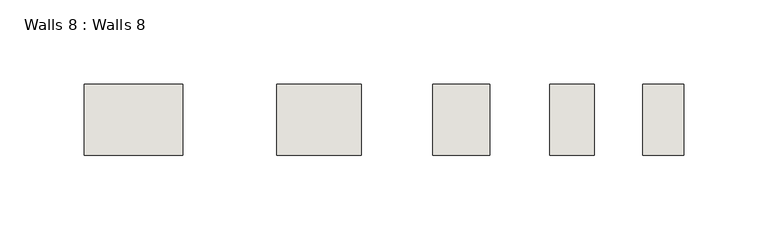
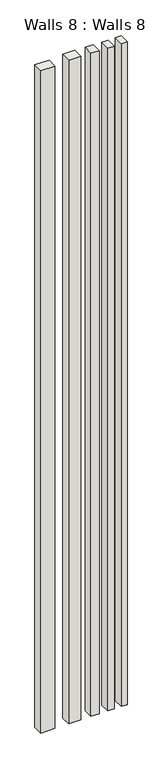
"""IFC4 building model written with IfcOpenShell, lengths in millimetres: wall geometry, Walls 8 : Walls 8."""

from ifc_helpers import new_model, si_unit, frame, origin, place, context, project, spatial, polyline, outline, extrude, source, transform, mapped, element, save


def walls_8_walls_8_e14edf94(model_context):
    return source(origin(), model_context, "Body", "SweptSolid", [
        extrude(outline(polyline([(-6662.2743282, -7775.4794447), (-6686.7552794, -7775.4794447), (-6686.7552794, -7733.3103215), (-6662.2743282, -7733.3103215), (-6662.2743282, -7775.4794447)])), frame((0.0, 0.0, 2899.4015195), z_axis=(0.0, 0.0, 1.0), x_axis=(1.0, 0.0, 0.0)), (0.0, 0.0, 1.0), 2896.3755776),
        extrude(outline(polyline([(-6715.5251751, -7775.4794447), (-6742.0237634, -7775.4794447), (-6742.0237634, -7733.3103215), (-6715.5251751, -7733.3103215), (-6715.5251751, -7775.4794447)])), frame((0.0, 0.0, 2899.4015195), z_axis=(0.0, 0.0, 1.0), x_axis=(1.0, 0.0, 0.0)), (0.0, 0.0, 1.0), 2895.7172276),
        extrude(outline(polyline([(-6777.6075818, -7775.4794447), (-6811.6771952, -7775.4794447), (-6811.6771952, -7733.3103215), (-6777.6075818, -7733.3103215), (-6777.6075818, -7775.4794447)])), frame((0.0, 0.0, 2899.4015195), z_axis=(0.0, 0.0, 1.0), x_axis=(1.0, 0.0, 0.0)), (0.0, 0.0, 1.0), 2897.6922776),
        extrude(outline(polyline([(-6854.0508605, -7775.4794447), (-6904.3695881, -7775.4794447), (-6904.3695881, -7733.3103215), (-6854.0508605, -7733.3103215), (-6854.0508605, -7775.4794447)])), frame((0.0, 0.0, 2899.4015195), z_axis=(0.0, 0.0, 1.0), x_axis=(1.0, 0.0, 0.0)), (0.0, 0.0, 1.0), 2900.2745688),
        extrude(outline(polyline([(-6960.3008412, -7775.4794447), (-7018.8954874, -7775.4794447), (-7018.8954874, -7733.3103215), (-6960.3008412, -7733.3103215), (-6960.3008412, -7775.4794447)])), frame((0.0, 0.0, 2899.4015195), z_axis=(0.0, 0.0, 1.0), x_axis=(1.0, 0.0, 0.0)), (0.0, 0.0, 1.0), 2894.113979),
    ])


if __name__ == "__main__":
    model = new_model("IFC4")
    model_context = context("Model", 3, world=origin())
    ifc_project = project(units=[si_unit("LENGTHUNIT", "METRE", prefix="MILLI")], contexts=[model_context])
    site = spatial("IfcSite", under=ifc_project)
    building = spatial("IfcBuilding", under=site)
    placement = place(None, origin())
    walls_8_walls_8_shape = walls_8_walls_8_e14edf94(model_context)
    element("IfcWall", 1, ObjectType="Walls 8 : Walls 8", at=placement, inside=building, context=model_context, shape_type="MappedRepresentation", body=[
        mapped(walls_8_walls_8_shape, transform((0.0, 0.0, 0.0), x_axis=(1.0, 0.0, 0.0), y_axis=(0.0, 1.0, 0.0), z_axis=(0.0, 0.0, 1.0))),
    ])
    save(model, "model.ifc")

# Revit data of these elements
# Element 1 (IfcWall, "Walls 8 : Walls 8")
#   Materials on its faces: "Default Wall"
# Materials
#   "Default Wall": colour RGB 80 80 80, transparency 0
